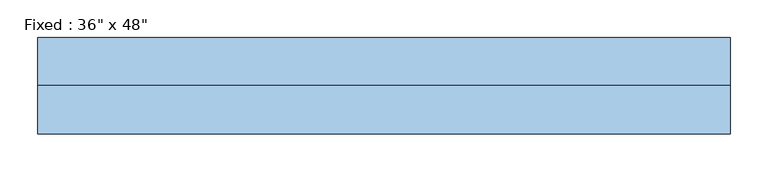
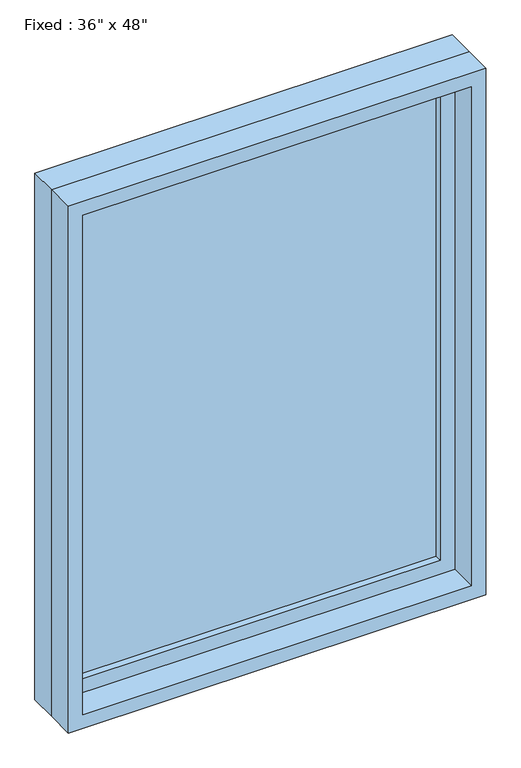
"""IFC4 building model written with IfcOpenShell, lengths in millimetres: window geometry."""

from ifc_helpers import new_model, si_unit, frame, origin, place, context, project, spatial, polyline, outline, extrude, source, transform, mapped, element, save


def window_1bec9dad(model_context):
    return source(origin(), model_context, "Body", "SweptSolid", [
        extrude(outline(polyline([(355.6, 15.875), (-431.8, 15.875), (-431.8, 28.575), (355.6, 28.575), (355.6, 15.875)])), frame((0.0, 0.0, 977.9), z_axis=(0.0, 0.0, 1.0), x_axis=(1.0, 0.0, 0.0)), (0.0, 0.0, 1.0), 1092.2),
        extrude(outline(polyline([(2114.55, -476.25), (933.45, -476.25), (933.45, 400.05), (2114.55, 400.05), (2114.55, -476.25)]), holes=[polyline([(2070.1, -431.8), (2070.1, 355.6), (977.9, 355.6), (977.9, -431.8), (2070.1, -431.8)])]), frame((0.0, 0.0, 0.0), z_axis=(0.0, 1.0, 0.0), x_axis=(0.0, 0.0, 1.0)), (0.0, 0.0, 1.0), 44.45),
        extrude(outline(polyline([(2133.6, -495.3), (914.4, -495.3), (914.4, 419.1), (2133.6, 419.1), (2133.6, -495.3)]), holes=[polyline([(2101.85, -463.55), (2101.85, 387.35), (946.15, 387.35), (946.15, -463.55), (2101.85, -463.55)])]), frame((0.0, -63.5, 0.0), z_axis=(0.0, 1.0, 0.0), x_axis=(0.0, 0.0, 1.0)), (0.0, 0.0, 1.0), 63.5),
        extrude(outline(polyline([(2133.6, 419.1), (2133.6, -495.3), (914.4, -495.3), (914.4, 419.1), (2133.6, 419.1)]), holes=[polyline([(2114.55, 400.05), (933.45, 400.05), (933.45, -476.25), (2114.55, -476.25), (2114.55, 400.05)])]), frame((0.0, 0.0, 0.0), z_axis=(0.0, 1.0, 0.0), x_axis=(0.0, 0.0, 1.0)), (0.0, 0.0, 1.0), 63.5),
    ])


if __name__ == "__main__":
    model = new_model("IFC4")
    model_context = context("Model", 3, world=origin())
    ifc_project = project(units=[si_unit("LENGTHUNIT", "METRE", prefix="MILLI")], contexts=[model_context])
    site = spatial("IfcSite", under=ifc_project)
    building = spatial("IfcBuilding", under=site)
    placement = place(None, origin())
    window_shape = window_1bec9dad(model_context)
    element("IfcWindow", 1, ObjectType="Fixed : 36\" x 48\"", at=placement, inside=building, context=model_context, shape_type="MappedRepresentation", body=[
        mapped(window_shape, transform((0.0, 0.0, 0.0), x_axis=(1.0, 0.0, 0.0), y_axis=(0.0, 1.0, 0.0), z_axis=(0.0, 0.0, 1.0))),
    ])
    save(model, "model.ifc")

# Revit data of these elements
# Type "Fixed : 36\" x 48\""
#   Type Mark = "W1"
#   Construction Type Id = "GSP4R"
#   Assembly Code = "B2020100"
#   Analytic Construction = "1/8 in Pilkington single glazing"
#   Visual Light Transmittance = 0.9
#   Solar Heat Gain Coefficient = 0.78
#   Heat Transfer Coefficient (U) = 0.6496 BTU/(h·ft²·°F)
#   Height = 4' - 0"
#   Default Sill Height = 3' - 0"
#   Width = 3' - 0"
#   Window Inset = 0' - 0 3/4"
#   Define Thermal Properties by = 1
#   Define Thermal Properties by = 1
#   Glass Pane Material = Glass
#   Sash Material = Sash
#   Wall Closure = (empty or 0)
# Element 1 (IfcWindow, "Fixed : 36\" x 48\"")
#   Materials on its faces: "Sash", "Glass"
# Materials
#   "Glass": class "Glass", colour RGB 0 128 192, transparency 0.75, Description = "Soda Lime Glass", Cost = 0
#   "Sash": class "Wood", colour RGB 224 178 126, transparency 0, Cost = 0
